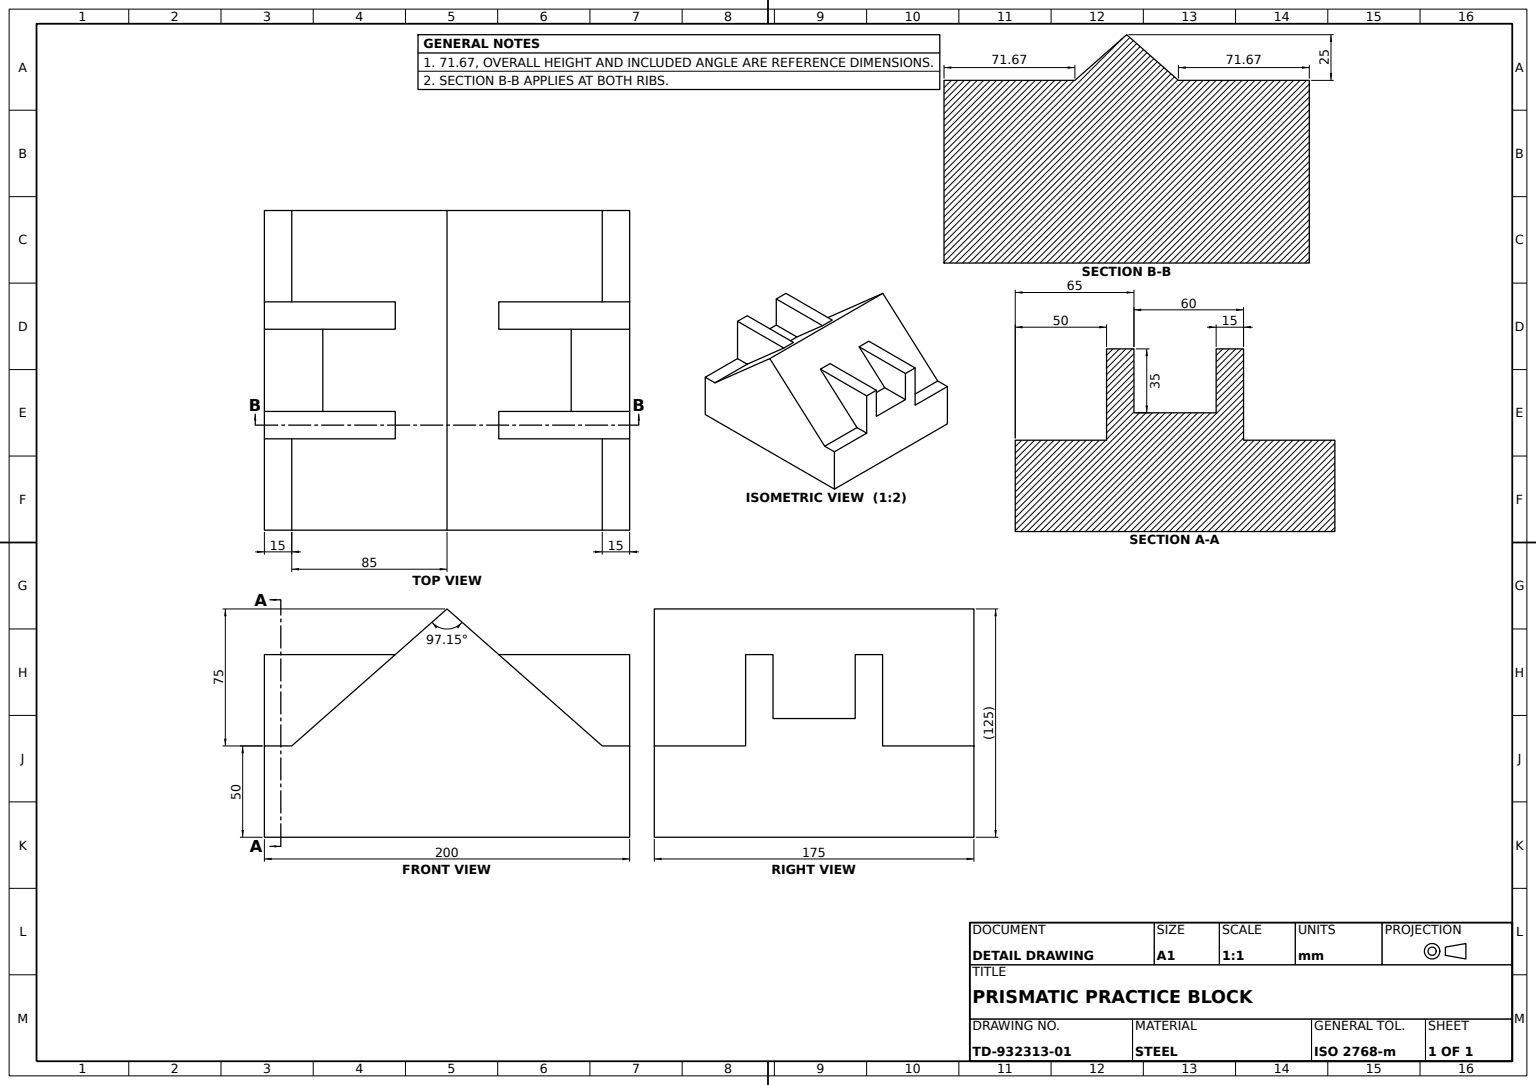
from build123d import *

# Parameters (mm, degrees)
BASE_BLOCK_PROFILE_W   = 200
BASE_BLOCK_PROFILE_H   = 175
BASE_BLOCK_DEPTH       = 50
NOTCHED_BOSS_175_DEPTH = 175
NOTCHED_BOSS_200_DEPTH = 200


with BuildPart() as part:
    # Base Block Profile → Base Block (new body)
    with BuildSketch(Plane.XY):
        with Locations((100, 87.5)):
            Rectangle(BASE_BLOCK_PROFILE_W, BASE_BLOCK_PROFILE_H)
    extrude(amount=-BASE_BLOCK_DEPTH)

    # Notched Boss Profile 175 → Notched Boss 175 (add)
    with BuildSketch(Plane.XZ):
        Polygon((100, 75), (15, 0), (185, 0), align=None)
    extrude(amount=-NOTCHED_BOSS_175_DEPTH)

    # Notched Boss Profile 200 → Notched Boss 200 (add)
    with BuildSketch(Plane(origin=(200, 0, 0), x_dir=(0, 0, -1), z_dir=(1, 0, 0))):
        Polygon((0, 50), (0, 125), (-50, 125), (-50, 110), (-15, 110), (-15, 65), (-50, 65), (-50, 50), (-15, 50), align=None)
    extrude(amount=-NOTCHED_BOSS_200_DEPTH)


solid = part.part
